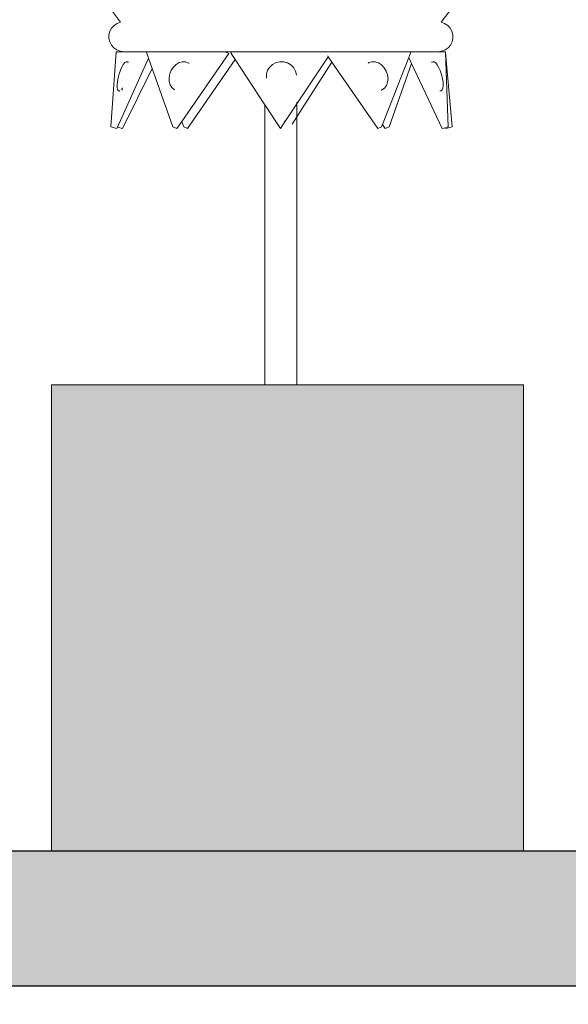
# Model space of a CAD drawing. Units: millimetres. Extents: x 7894 to 8038, y 6851 to 6951.
# Tile 21 of 49: x 7956.664 to 7958.696, y 6906.405 to 6910.053. Entities that reach past the tile are written whole.
import ezdxf

# ---------------------------------------------------------------- set-up
doc = ezdxf.new("R2010")
doc.units = ezdxf.units.MM
for name, color, linetype, lineweight in [('A-ANNO-DIMS', 2, 'Continuous', 18), ('A-FURN-ACCS', 8, 'Continuous', 13), ('A-FURN-SHLF', 7, 'Continuous', 30)]:
    doc.layers.add(name, color=color, linetype=linetype, lineweight=lineweight)
doc.layers.add('A-FURN-ACCS-PATT', color=116, linetype='Continuous', lineweight=9, true_color=0x136734)
doc.layers.add('A-FURN-PATT', color=32, linetype='Continuous', lineweight=9, true_color=0xcd6928)
doc.styles.get("Standard").update_dxf_attribs({"font": 'arial.ttf'})
doc.dimstyles.new('ISO-25', dxfattribs={"dimtxt": 1, "dimasz": 1, "dimexe": 1.25, "dimexo": 0.625, "dimtad": 1, "dimdec": 0, "dimlunit": 4, "dimtxsty": 'Standard', "dimcen": 2.5, "dimclrt": 1, "dimadec": 0, "dimazin": 0, "dimtfac": 1, "dimtdec": 0, "dimtmove": 0, "dimatfit": 3, "dimfxl": 1, "dimarcsym": 0})

# ---------------------------------------------------------------- blocks, each defined once
blk = doc.blocks.new('DISPLAY-LEAF-FINIAL')
for p, q in [((0.2072, 1.3429), (0, 1.6201)), ((1.6021, 1.6201), (1.395, 1.3429)), ((0.1678, 1.3095), (0.1742, 1.3213)), ((0.1742, 1.3213), (0.1833, 1.3311)), ((0.1833, 1.3311), (0.1945, 1.3384)), ((0.1945, 1.3384), (0.2072, 1.3429)), ((1.395, 1.3429), (1.4076, 1.3384)), ((1.4076, 1.3384), (1.4188, 1.3311)), ((1.4188, 1.3311), (1.4279, 1.3213)), ((1.4279, 1.3213), (1.4344, 1.3095)), ((0.1641, 1.2831), (0.1643, 1.2966)), ((0.1672, 1.2701), (0.1641, 1.2831)), ((0.1643, 1.2966), (0.1678, 1.3095)), ((1.4344, 1.3095), (1.4378, 1.2966)), ((1.438, 1.2831), (1.435, 1.2701)), ((1.4378, 1.2966), (1.438, 1.2831)), ((0.1733, 1.2582), (0.1672, 1.2701)), ((0.1821, 1.2481), (0.1733, 1.2582)), ((0.1931, 1.2404), (0.1821, 1.2481)), ((0.2056, 1.2356), (0.1931, 1.2404)), ((1.4091, 1.2404), (1.3965, 1.2356)), ((1.42, 1.2481), (1.4091, 1.2404)), ((1.4288, 1.2582), (1.42, 1.2481)), ((1.435, 1.2701), (1.4288, 1.2582)), ((0.1714, 0.9553), (0.1907, 1.234)), ((0.2189, 1.234), (0.1907, 1.234)), ((0.1964, 0.9543), (0.3109, 1.2098)), ((0.2189, 1.234), (0.2056, 1.2356)), ((0.2189, 1.234), (0.2969, 1.234)), ((0.2969, 1.234), (0.3023, 1.234)), ((0.3029, 1.2321), (0.2969, 1.234)), ((0.3029, 1.2321), (0.3023, 1.234)), ((0.3023, 1.234), (0.5943, 1.234)), ((0.3109, 1.2098), (0.3029, 1.2321)), ((0.3244, 1.1717), (0.3109, 1.2098)), ((0.434, 0.9751), (0.6087, 1.2276)), ((0.455, 0.949), (0.6322, 1.205)), ((0.5943, 1.234), (0.6175, 1.234)), ((0.6087, 1.2276), (0.5943, 1.234)), ((0.6175, 1.2276), (0.6175, 1.234)), ((0.9517, 1.234), (0.6175, 1.234)), ((0.6322, 1.205), (0.6175, 1.2276)), ((0.7416, 1.0372), (0.6322, 1.205)), ((0.8605, 1.0411), (0.9765, 1.2154)), ((0.9809, 1.2337), (0.9517, 1.234)), ((0.9765, 1.2154), (0.9744, 1.2185)), ((0.9902, 1.1955), (0.9765, 1.2154)), ((0.9809, 1.2337), (0.9815, 1.234)), ((0.9815, 1.234), (0.983, 1.234)), ((1.2836, 1.234), (0.983, 1.234)), ((1.1768, 0.964), (1.2748, 1.2121)), ((1.2748, 1.2121), (1.2826, 1.2319)), ((1.285, 1.1903), (1.2748, 1.2121)), ((1.2826, 1.2319), (1.2898, 1.234)), ((1.2826, 1.2319), (1.2836, 1.234)), ((1.2836, 1.234), (1.2898, 1.234)), ((1.2898, 1.234), (1.3832, 1.234)), ((1.3965, 1.2356), (1.3832, 1.234)), ((1.41, 1.2337), (1.3832, 1.234)), ((1.4111, 1.234), (1.41, 1.2337)), ((1.4113, 1.2316), (1.4111, 1.234)), ((1.4348, 0.9553), (1.4113, 1.2316)), ((1.4203, 0.9553), (1.4113, 1.2316)), ((0.2065, 1.165), (0.2118, 1.177)), ((0.2118, 1.177), (0.2173, 1.1867)), ((0.2147, 0.949), (0.3244, 1.1717)), ((0.2173, 1.1867), (0.2227, 1.1934)), ((0.2227, 1.1934), (0.2276, 1.1967)), ((0.2276, 1.1967), (0.2317, 1.1963)), ((0.2325, 1.1953), (0.2317, 1.1963)), ((0.2325, 1.1953), (0.2366, 1.1949)), ((0.4015, 0.9553), (0.3244, 1.1717)), ((0.3948, 1.165), (0.4028, 1.177)), ((0.4028, 1.177), (0.4128, 1.1867)), ((0.4128, 1.1867), (0.4241, 1.1934)), ((0.4241, 1.1934), (0.436, 1.1967)), ((0.436, 1.1967), (0.4475, 1.1963)), ((0.4475, 1.1963), (0.4584, 1.1919)), ((0.4584, 1.1919), (0.4611, 1.1909)), ((0.752, 1.165), (0.7597, 1.177)), ((0.7597, 1.177), (0.7703, 1.1867)), ((0.7703, 1.1867), (0.7831, 1.1934)), ((0.7831, 1.1934), (0.7973, 1.1967)), ((0.7973, 1.1967), (0.8119, 1.1963)), ((0.8119, 1.1963), (0.8259, 1.1923)), ((0.8259, 1.1923), (0.8383, 1.1849)), ((0.8383, 1.1849), (0.8484, 1.1746)), ((0.8484, 1.1746), (0.8553, 1.1622)), ((0.8605, 0.9923), (0.9902, 1.1955)), ((1.16, 0.949), (0.9902, 1.1955)), ((1.1241, 1.1921), (1.1257, 1.1925)), ((1.1257, 1.1925), (1.127, 1.1934)), ((1.127, 1.1934), (1.1382, 1.1967)), ((1.1382, 1.1967), (1.1502, 1.1963)), ((1.1502, 1.1963), (1.1624, 1.1923)), ((1.1624, 1.1923), (1.1737, 1.1849)), ((1.1737, 1.1849), (1.1835, 1.1746)), ((1.1835, 1.1746), (1.1911, 1.1622)), ((1.2015, 0.9553), (1.285, 1.1903)), ((1.398, 0.949), (1.285, 1.1903)), ((1.359, 1.1953), (1.3638, 1.1967)), ((1.359, 1.1953), (1.3619, 1.1951)), ((1.3638, 1.1967), (1.3687, 1.1963)), ((1.3687, 1.1963), (1.3744, 1.1923)), ((1.3744, 1.1923), (1.3804, 1.1849)), ((1.3804, 1.1849), (1.3863, 1.1746)), ((1.3863, 1.1746), (1.3917, 1.1622)), ((0.1955, 1.1237), (0.1981, 1.1374)), ((0.1981, 1.1374), (0.2018, 1.1515)), ((0.2018, 1.1515), (0.2065, 1.165)), ((0.3867, 1.1374), (0.3893, 1.1515)), ((0.3871, 1.1237), (0.3867, 1.1374)), ((0.3893, 1.1515), (0.3948, 1.165)), ((0.7474, 1.1361), (0.7475, 1.1373)), ((0.7475, 1.1373), (0.7478, 1.1515)), ((0.7478, 1.1515), (0.752, 1.165)), ((0.8553, 1.1622), (0.8587, 1.1485)), ((0.8587, 1.1471), (0.8587, 1.1485)), ((1.1911, 1.1622), (1.196, 1.1485)), ((1.196, 1.1485), (1.1978, 1.1344)), ((1.1978, 1.1344), (1.1964, 1.1209)), ((1.3917, 1.1622), (1.3963, 1.1485)), ((1.3963, 1.1485), (1.3997, 1.1344)), ((1.3997, 1.1344), (1.4018, 1.1209)), ((0.1943, 1.1113), (0.1955, 1.1237)), ((0.1946, 1.101), (0.1943, 1.1113)), ((0.1963, 1.0936), (0.1946, 1.101)), ((0.2112, 1.0961), (0.2129, 1.0925)), ((0.2141, 1.1), (0.2145, 1.0978)), ((0.3906, 1.1113), (0.3871, 1.1237)), ((0.3969, 1.101), (0.3906, 1.1113)), ((0.4056, 1.0936), (0.3969, 1.101)), ((1.1847, 1.0992), (1.1752, 1.0925)), ((1.192, 1.1089), (1.1847, 1.0992)), ((1.1964, 1.1209), (1.192, 1.1089)), ((1.4012, 1.0992), (1.3987, 1.0925)), ((1.4023, 1.1089), (1.4012, 1.0992)), ((1.4018, 1.1209), (1.4023, 1.1089)), ((0.1993, 1.0896), (0.1963, 1.0936)), ((0.2034, 1.0892), (0.1993, 1.0896)), ((0.2041, 1.0883), (0.2034, 1.0892)), ((0.2129, 1.0925), (0.2137, 1.0919)), ((0.4087, 1.0923), (0.4056, 1.0936)), ((1.1736, 1.092), (1.1723, 1.0911)), ((1.1736, 1.092), (1.1752, 1.0925)), ((1.3919, 1.0894), (1.39, 1.0879)), ((1.39, 1.0879), (1.3948, 1.0892)), ((1.3987, 1.0925), (1.3948, 1.0892)), ((0.7416, 0), (0.7416, 1.0372)), ((0.7992, 0.949), (0.7416, 1.0372)), ((0.8158, 0.974), (0.8605, 1.0411)), ((0.8605, 1.0411), (0.8605, 1.0475)), ((0.8605, 0.9923), (0.8605, 1.0411)), ((0.8431, 0.9651), (0.8605, 0.9923)), ((0.8605, 0), (0.8605, 0.9923)), ((0.1941, 0.949), (0.1714, 0.9553)), ((0.1941, 0.949), (0.1964, 0.9543)), ((0.2147, 0.949), (0.1964, 0.9543)), ((0.4159, 0.949), (0.4015, 0.9553)), ((0.4159, 0.949), (0.434, 0.9751)), ((0.4421, 0.9553), (0.434, 0.9751)), ((0.455, 0.949), (0.4421, 0.9553)), ((0.7992, 0.949), (0.8158, 0.974)), ((0.8158, 0.974), (0.8137, 0.9772)), ((0.8165, 0.9731), (0.8158, 0.974)), ((1.16, 0.949), (1.1734, 0.9553)), ((1.1734, 0.9553), (1.1768, 0.964)), ((1.1872, 0.949), (1.1768, 0.964)), ((1.1872, 0.949), (1.2015, 0.9553)), ((1.398, 0.949), (1.4105, 0.9525)), ((1.4105, 0.9525), (1.4203, 0.9553)), ((1.412, 0.949), (1.4105, 0.9525)), ((1.412, 0.949), (1.4348, 0.9553))]:
    blk.add_line(p, q)
blk = doc.blocks.new('*D23')
at = {"layer": 'A-ANNO-DIMS', "color": 0, "lineweight": -2, "transparency": 16777216}
for p, q in [((7940.0888, 6907.098), (7940.0888, 6947.7928)), ((7971.9356, 6928.989), (7971.9356, 6947.7928)), ((7941.0888, 6946.5428), (7970.9356, 6946.5428))]:
    blk.add_line(p, q, dxfattribs=at)
at = {"layer": 'A-ANNO-DIMS', "color": 0, "transparency": 16777216}
for points in [[(7941.0888, 6946.7095), (7941.0888, 6946.3762), (7940.0888, 6946.5428)], [(7970.9356, 6946.7095), (7970.9356, 6946.3762), (7971.9356, 6946.5428)]]:
    blk.add_solid(points, dxfattribs=at)
at = {"layer": 'Defpoints', "color": 0, "transparency": 16777216}
for p in [(7971.9356, 6946.5428), (7971.9356, 6928.364), (7940.0888, 6906.473)]:
    blk.add_point(p, dxfattribs=at)
at = {"layer": 'A-ANNO-DIMS', "color": 1, "transparency": 16777216, "insert": (7956.0122, 6947.6784), "char_height": 1, "attachment_point": 5}
blk.add_mtext('2\'-8"', dxfattribs=at)
blk = doc.blocks.new('*D25')
at = {"layer": 'A-ANNO-DIMS', "color": 0, "lineweight": -2, "transparency": 16777216}
for p, q in [((7940.0888, 6905.848), (7940.0888, 6903.2865)), ((7964.3408, 6905.8484), (7964.3408, 6903.2865)), ((7941.0888, 6904.5365), (7963.3408, 6904.5365))]:
    blk.add_line(p, q, dxfattribs=at)
at = {"layer": 'A-ANNO-DIMS', "color": 0, "transparency": 16777216}
for points in [[(7941.0888, 6904.7032), (7941.0888, 6904.3699), (7940.0888, 6904.5365)], [(7963.3408, 6904.7032), (7963.3408, 6904.3699), (7964.3408, 6904.5365)]]:
    blk.add_solid(points, dxfattribs=at)
at = {"layer": 'Defpoints', "color": 0, "transparency": 16777216}
for p in [(7940.0888, 6906.473), (7964.3408, 6906.4734), (7964.3408, 6904.5365)]:
    blk.add_point(p, dxfattribs=at)
at = {"layer": 'A-ANNO-DIMS', "color": 1, "transparency": 16777216, "insert": (7952.2148, 6905.6786), "char_height": 1, "attachment_point": 5}
blk.add_mtext('2\'-0 1/2"', dxfattribs=at)
blk = doc.blocks.new('*D26')
at = {"layer": 'A-ANNO-DIMS', "color": 0, "lineweight": -2, "transparency": 16777216}
for p, q in [((7950.9654, 6918.7198), (7975.2272, 6918.7198)), ((7973.9772, 6917.7198), (7973.9772, 6907.4734)), ((7964.9658, 6906.4734), (7975.2272, 6906.4734))]:
    blk.add_line(p, q, dxfattribs=at)
at = {"layer": 'A-ANNO-DIMS', "color": 0, "transparency": 16777216}
for points in [[(7973.8105, 6917.7198), (7974.1439, 6917.7198), (7973.9772, 6918.7198)], [(7973.8105, 6907.4734), (7974.1439, 6907.4734), (7973.9772, 6906.4734)]]:
    blk.add_solid(points, dxfattribs=at)
at = {"layer": 'Defpoints', "color": 0, "transparency": 16777216}
for p in [(7950.3404, 6918.7198), (7964.3408, 6906.4734), (7973.9772, 6906.4734)]:
    blk.add_point(p, dxfattribs=at)
at = {"layer": 'A-ANNO-DIMS', "color": 1, "transparency": 16777216, "insert": (7972.8416, 6912.5966), "char_height": 1, "attachment_point": 5, "rotation": 90}
blk.add_mtext('1\'-0"', dxfattribs=at)

msp = doc.modelspace()

# ---------------------------------------------------------------- hatches: boundary and pattern name
at = {"layer": 'A-FURN-ACCS-PATT'}
h = msp.add_hatch(color=256, dxfattribs=at)
h.dxf.hatch_style = 1
h.paths.add_polyline_path([(7947.5161, 6931.8853), (7946.6774, 6931.8853), (7946.5585, 6931.8853), (7945.7683, 6931.8853), (7945.7683, 6930.1581), (7947.5161, 6930.1581)])
h.paths.add_polyline_path([(7947.4851, 6922.447), (7946.6464, 6922.447), (7946.5276, 6922.447), (7945.7373, 6922.447), (7945.7373, 6920.7198), (7947.4851, 6920.7198)])
h.paths.add_polyline_path([(7968.0212, 6935.881), (7967.1825, 6935.881), (7967.0637, 6935.881), (7966.2734, 6935.881), (7966.2734, 6934.1538), (7968.0212, 6934.1538)])
h.paths.add_polyline_path([(7960.6099, 6924.8555), (7959.7712, 6924.8555), (7959.6523, 6924.8555), (7958.862, 6924.8555), (7958.862, 6923.1283), (7960.6099, 6923.1283)])
h.paths.add_polyline_path([(7964.717, 6924.8555), (7963.8783, 6924.8555), (7963.7594, 6924.8555), (7962.9691, 6924.8555), (7962.9691, 6923.1283), (7964.717, 6923.1283)])
h.paths.add_polyline_path([(7971.0698, 6924.8555), (7970.2311, 6924.8555), (7970.1123, 6924.8555), (7969.322, 6924.8555), (7969.322, 6923.1283), (7971.0698, 6923.1283)])
h.paths.add_polyline_path([(7958.5294, 6908.7006), (7957.6907, 6908.7006), (7957.5718, 6908.7006), (7956.7815, 6908.7006), (7956.7815, 6906.9734), (7958.5294, 6906.9734)])
at = {"layer": 'A-FURN-PATT'}
h = msp.add_hatch(color=256, dxfattribs=at)
h.dxf.hatch_style = 1
h.paths.add_polyline_path([(7942.8406, 6913.3629), (7942.8593, 6913.356), (7942.8677, 6913.356), (7942.8677, 6914.2132), (7942.876, 6914.2376), (7942.8813, 6914.2376), (7942.9022, 6914.2457), (7943.3657, 6914.2457), (7943.3844, 6914.2376), (7943.3861, 6914.2376), (7943.3858, 6914.2132), (7943.3852, 6913.2312), (7943.3944, 6906.9948), (7943.387, 6906.9732), (7943.4027, 6906.9732), (7943.403, 6906.9948), (7943.4029, 6908.4372), (7943.3944, 6914.2132), (7943.4169, 6914.2376), (7943.4198, 6914.2457), (7943.4555, 6914.2457), (7943.4603, 6914.238), (7943.8607, 6914.2452), (7943.8615, 6914.2457), (7943.8623, 6914.2452), (7943.8866, 6914.2457), (7943.8944, 6914.2402), (7943.9104, 6914.2376), (7943.9211, 6914.2132), (7943.9294, 6914.2376), (7943.9318, 6914.2376), (7943.9453, 6914.2398), (7943.9488, 6914.2457), (7943.9797, 6914.2452), (7943.9807, 6914.2457), (7943.9815, 6914.2451), (7944.3738, 6914.2376), (7944.3882, 6914.2457), (7944.4201, 6914.2457), (7944.4341, 6914.2376), (7944.4395, 6914.2376), (7944.4478, 6914.2132), (7944.4478, 6914.1031), (7944.4622, 6914.099), (7944.7359, 6914.1607), (7944.8923, 6914.2014), (7944.9541, 6914.2098), (7944.955, 6914.21), (7946.556, 6907.1325), (7946.5534, 6907.1122), (7946.5529, 6907.1152), (7946.499, 6907.103), (7946.3343, 6907.0604), (7946.0282, 6906.9914), (7945.6731, 6908.5712), (7944.4484, 6914.0015), (7944.4478, 6906.9948), (7944.4404, 6906.9732), (7947.0373, 6906.9734), (7964.3408, 6906.9734), (7964.3408, 6906.4734), (7947.0373, 6906.4734), (7940.0888, 6906.473), (7940.0888, 6906.973), (7941.9951, 6906.9731), (7941.9899, 6906.9898), (7941.9899, 6913.3353), (7941.9968, 6913.3574), (7942.003, 6913.3571), (7942.0169, 6913.3629), (7942.0366, 6913.3629), (7942.0378, 6913.3629), (7942.0479, 6913.356), (7942.8142, 6913.356), (7942.8157, 6913.356), (7942.8346, 6913.356)])
h.paths.add_polyline_path([(7942.8598, 6913.0201), (7942.861, 6913.3353), (7942.8677, 6906.9948), (7942.876, 6906.9759), (7942.876, 6906.9903), (7942.8813, 6914.2376), (7942.876, 6914.2321), (7942.876, 6914.2177), (7942.8809, 6906.9647), (7942.8784, 6906.9704), (7942.876, 6906.9704), (7942.8574, 6906.9704), (7942.8613, 6911.8549)], flags=16)
h.paths.add_polyline_path([(7942.8613, 6911.8549), (7942.8677, 6906.9948), (7942.8686, 6906.9921), (7942.8677, 6906.9898), (7942.8616, 6906.9704), (7942.8598, 6906.9704), (7942.8574, 6906.9704), (7942.0002, 6906.9704), (7941.9978, 6906.9704), (7941.996, 6906.9704), (7941.9899, 6906.9898), (7941.9978, 6906.9704), (7942.0002, 6906.9704), (7942.8598, 6906.9704), (7942.8616, 6906.9748)], flags=16)
h.paths.add_polyline_path([(7942.023, 6913.356), (7942.0169, 6913.3629), (7942.0366, 6913.3629), (7942.0378, 6913.3629), (7942.0367, 6913.3614), (7942.0369, 6913.356)], flags=16)
h.paths.add_polyline_path([(7942.0366, 6913.3629), (7942.0169, 6913.3629), (7942.0196, 6913.3598)], flags=0)
h.paths.add_polyline_path([(7942.0353, 6913.356), (7942.0369, 6913.356), (7942.0367, 6913.3614)], flags=0)
h.paths.add_polyline_path([(7943.9293, 6906.9759), (7943.9211, 6906.9948), (7943.9294, 6906.9704)], flags=0)
h.paths.add_polyline_path([(7943.9125, 6914.2132), (7943.8982, 6914.2376), (7943.8944, 6914.2402), (7943.8832, 6914.2421), (7943.8781, 6914.2367), (7943.8765, 6914.2376), (7943.8789, 6914.2376), (7943.8866, 6914.2457), (7943.8623, 6914.2452), (7943.8607, 6914.2452), (7943.8615, 6914.2457), (7943.8623, 6914.2452), (7943.8866, 6914.2457), (7943.8944, 6914.2402), (7943.8982, 6914.2376), (7943.9097, 6914.218), (7943.9125, 6914.2168), (7943.9079, 6906.9704), (7943.9104, 6906.9704), (7943.9211, 6914.2132), (7943.9294, 6914.2376), (7943.9318, 6914.2376), (7943.9453, 6914.2398), (7943.9488, 6914.2457), (7943.9797, 6914.2452), (7943.9807, 6914.2457), (7943.9815, 6914.2451), (7944.3738, 6914.2376), (7944.3882, 6914.2457), (7944.4201, 6914.2457), (7944.4341, 6914.2376), (7944.4395, 6914.2376), (7944.4395, 6914.2177), (7944.4341, 6914.0941), (7944.4478, 6914.1004), (7944.4513, 6914.1021), (7944.4622, 6914.099), (7944.4343, 6914.0927), (7944.429, 6914.0915), (7944.4341, 6914.069), (7944.4484, 6914.0015), (7944.4341, 6914.0649), (7944.4346, 6906.9704), (7944.4371, 6906.9704), (7944.4395, 6906.9759), (7944.4395, 6906.9704), (7943.931, 6906.9704), (7943.9128, 6906.9704), (7943.9079, 6906.9704)], flags=16)
h.paths.add_polyline_path([(7943.9211, 6914.2132), (7943.9294, 6914.2376), (7943.9318, 6914.2376), (7943.9453, 6914.2398), (7943.9488, 6914.2457), (7943.9797, 6914.2452), (7943.9807, 6914.2457), (7943.9815, 6914.2451), (7944.3738, 6914.2376), (7944.3882, 6914.2457), (7944.4201, 6914.2457), (7944.4321, 6914.2387), (7944.4249, 6914.2376), (7944.4041, 6914.2376), (7944.4032, 6914.2136), (7944.4032, 6914.2376), (7944.4025, 6914.2379), (7944.3897, 6914.2382), (7944.3753, 6914.2384), (7944.3738, 6914.2376), (7943.9815, 6914.2451), (7943.9488, 6914.2457), (7943.9453, 6914.2398), (7943.9294, 6914.2132), (7943.931, 6906.9721), (7943.931, 6906.9704), (7943.9294, 6906.9704), (7943.9293, 6906.9759), (7943.9294, 6914.2132), (7943.9439, 6914.2376), (7943.9318, 6914.2376)], flags=0)
h.paths.add_polyline_path([(7942.8813, 6914.2376), (7942.8778, 6914.2362), (7942.8796, 6914.2404), (7942.885, 6914.239)], flags=17)
h.paths.add_polyline_path([(7944.4116, 6914.242), (7944.4104, 6914.2408), (7944.4125, 6914.2418)], flags=0)
h.paths.add_polyline_path([(7944.3879, 6914.2382), (7944.3882, 6914.2457), (7944.4094, 6914.241), (7944.4103, 6914.2408), (7944.4036, 6914.2373), (7944.39, 6914.2447), (7944.3897, 6914.2382)], flags=0)
h.paths.add_polyline_path([(7963.1359, 6906.9526), (7963.1396, 6906.9526), (7963.1431, 6906.9582)], flags=16)
h.paths.add_polyline_path([(7954.3975, 6907.3902), (7954.397, 6907.3948), (7954.3984, 6907.4007), (7954.3975, 6907.567), (7954.3984, 6907.5978), (7954.3986, 6907.7694), (7954.3978, 6907.7989), (7954.399, 6907.8759), (7954.3992, 6907.9037), (7954.3944, 6907.9081), (7954.4019, 6907.9055), (7954.3996, 6907.93), (7954.3988, 6907.9307), (7954.3841, 6907.9429), (7946.6754, 6907.9429), (7946.6535, 6907.9232), (7946.6531, 6907.9127), (7946.6527, 6907.7694), (7946.6525, 6907.4007), (7946.653, 6907.1185), (7946.6574, 6907.1224), (7946.656, 6907.1145), (7946.6571, 6907.1135), (7946.6675, 6907.1209), (7946.7515, 6907.1209), (7946.9105, 6907.1209), (7954.3003, 6907.1209), (7954.3895, 6907.1209), (7954.3915, 6907.1191), (7954.3991, 6907.1209), (7954.399, 6907.1383), (7954.3978, 6907.2163), (7954.3986, 6907.2413)], flags=17)
h.paths.add_polyline_path([(7954.3003, 6907.1209), (7954.3003, 6907.1136), (7946.9105, 6907.1129), (7946.7516, 6907.1136), (7946.7515, 6907.1209), (7946.6675, 6907.1209), (7946.6531, 6907.1106), (7946.653, 6907.1185), (7946.6574, 6907.1224), (7946.656, 6907.1145), (7946.6571, 6907.1135), (7946.6675, 6907.1209), (7946.7515, 6907.1209), (7946.9105, 6907.1209)], flags=17)
h.paths.add_polyline_path([(7954.3981, 6907.9048), (7954.3944, 6907.9081), (7954.3997, 6907.9062), (7954.4007, 6907.9186), (7954.4019, 6907.9055), (7954.405, 6907.9072), (7954.4044, 6907.9046), (7954.4027, 6907.8974), (7954.4024, 6907.9009), (7954.3996, 6907.9034), (7954.3996, 6907.9025), (7954.3994, 6907.9023), (7954.3995, 6907.9035)], flags=17)

# ---------------------------------------------------------------- linework, layer by layer
at = {"layer": 'A-FURN-ACCS'}
for p, q in [((7956.7815, 6906.9734), (7956.7815, 6908.7006)), ((7956.7815, 6908.7006), (7957.5718, 6908.7006)), ((7957.6907, 6908.7006), (7957.5718, 6908.7006)), ((7957.6907, 6908.7006), (7958.5294, 6908.7006)), ((7958.5294, 6906.9734), (7958.5294, 6908.7006))]:
    msp.add_line(p, q, dxfattribs=at)
at = {"layer": 'A-FURN-SHLF'}
for p, q in [((7947.0373, 6906.9734), (7964.3408, 6906.9734)), ((7947.0373, 6906.4734), (7964.3408, 6906.4734))]:
    msp.add_line(p, q, dxfattribs=at)

# ---------------------------------------------------------------- block references
at = {"layer": 'A-FURN-ACCS'}
msp.add_blockref('DISPLAY-LEAF-FINIAL', (7956.8302, 6908.7006), dxfattribs=at)

# ---------------------------------------------------------------- dimensions: what is measured, and where the dimension line sits
at = {"layer": 'A-ANNO-DIMS'}
for base, p2, picture, middle in [((7971.9356, 6946.5428), (7971.9356, 6928.364), '*D23', (7956.0122, 6947.6784)), ((7964.3408, 6904.5365), (7964.3408, 6906.4734), '*D25', (7952.2148, 6905.6786))]:
    dim = msp.add_linear_dim(base=base, p1=(7940.0888, 6906.473), p2=p2, dimstyle='ISO-25', override={"dimdec": 1, "dimlfac": 1, "dimrnd": 0, "dimzin": 1, "dimdsep": 46, "dimlunit": 4, "dimfrac": 2}, dxfattribs=at)
    dim.commit()
    dim.dimension.update_dxf_attribs({"geometry": picture, "text_midpoint": middle})
dim = msp.add_linear_dim(base=(7973.9772, 6906.4734), p1=(7950.3404, 6918.7198), p2=(7964.3408, 6906.4734), angle=90, dimstyle='ISO-25', override={"dimdec": 1, "dimlfac": 1, "dimrnd": 0, "dimzin": 1, "dimdsep": 46, "dimlunit": 4, "dimfrac": 2}, dxfattribs=at)
dim.commit()
dim.dimension.update_dxf_attribs({"geometry": '*D26', "text_midpoint": (7972.8416, 6912.5966)})

doc.saveas('drawing.dxf')
